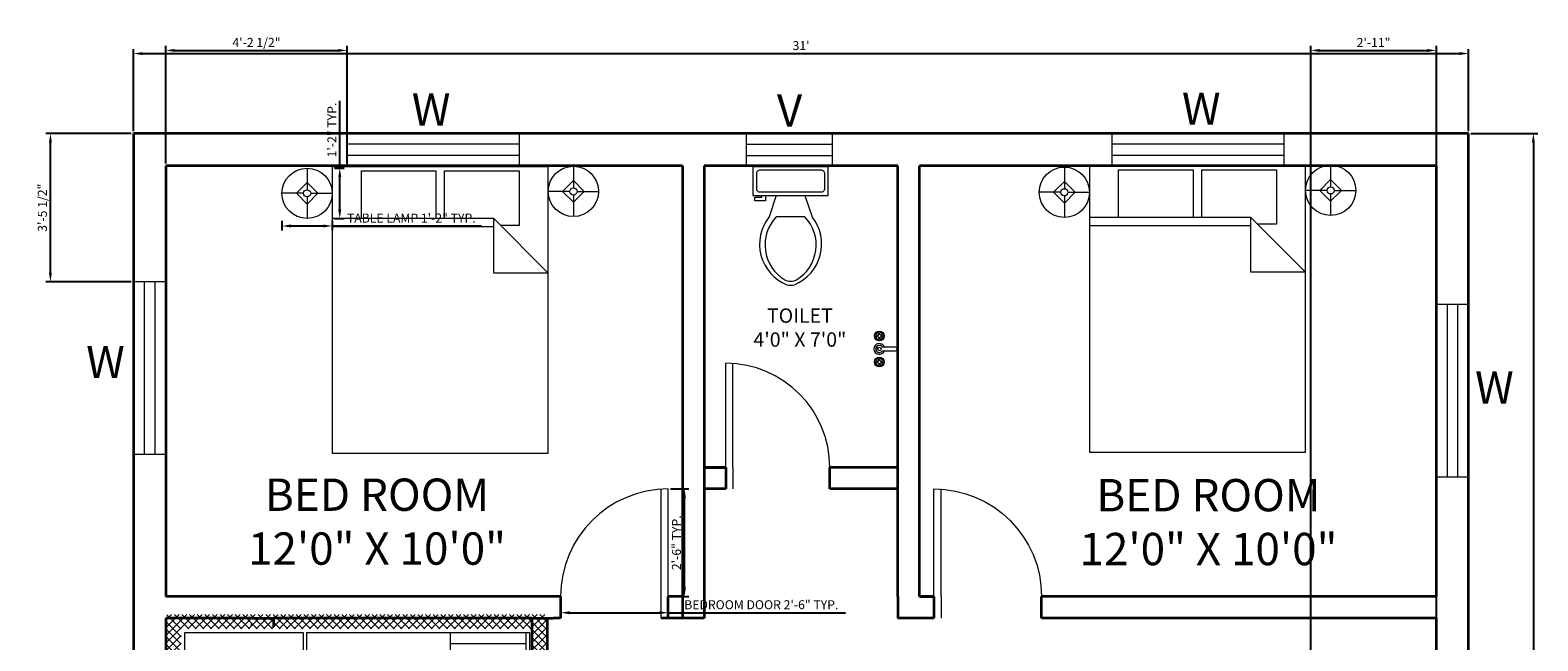
# Model space of a CAD drawing. Units: inches. Extents: x 1642 to 5612, y 1595 to 4064.
# Tile 6 of 6: x 2333 to 2754, y 1979 to 2149. Entities that reach past the tile are written whole.
import ezdxf

# ---------------------------------------------------------------- set-up
doc = ezdxf.new("R2010")
doc.units = ezdxf.units.IN
for name, color, linetype, lineweight in [('A-ANNO-DIMS', 2, 'Continuous', 18), ('A-ANNO-TEXT', 7, 'Continuous', 18), ('A-AREA-IDEN', 7, 'Continuous', 25), ('A-DOOR', 3, 'Continuous', 18), ('A-FLOR-FIXT', 9, 'Continuous', 18), ('A-FURN', 8, 'Continuous', 13), ('A-GLAZ', 4, 'Continuous', 18), ('A-WALL', 7, 'Continuous', 35)]:
    doc.layers.add(name, color=color, linetype=linetype, lineweight=lineweight)
doc.styles.get("Standard").update_dxf_attribs({"font": 'arial.ttf'})
doc.dimstyles.new('ISO-25', dxfattribs={"dimtxt": 2.5, "dimasz": 2.5, "dimexe": 1.25, "dimexo": 0.625, "dimtad": 1, "dimdec": 0, "dimlunit": 3, "dimtxsty": 'Standard', "dimcen": 2.5, "dimadec": 0, "dimazin": 0, "dimtfac": 1, "dimtdec": 0, "dimtmove": 0, "dimatfit": 3, "dimfxl": 1, "dimarcsym": 0})

# ---------------------------------------------------------------- blocks, each defined once
blk = doc.blocks.new('Kitchen Layout - 7 x 8 ft')
for p, q in [((-5, 81.32), (2.68, 89)), ((-5, 83.44), (0.56, 89)), ((-5, 85.56), (-1.56, 89)), ((-5, 87.68), (-3.68, 89)), ((-1, 84.97), (-5, 88.97)), ((1.09, 85), (-2.91, 89)), ((3.21, 85), (-0.79, 89)), ((0.81, 85), (4.81, 89)), ((5.34, 85), (1.34, 89)), ((2.93, 85), (6.93, 89)), ((7.46, 85), (3.46, 89)), ((5.05, 85), (9.05, 89)), ((9.58, 85), (5.58, 89)), ((7.17, 85), (11.17, 89)), ((11.7, 85), (7.7, 89)), ((9.29, 85), (13.29, 89)), ((13.82, 85), (9.82, 89)), ((11.41, 85), (15.41, 89)), ((15.94, 85), (11.94, 89)), ((13.53, 85), (17.53, 89)), ((18.06, 85), (14.06, 89)), ((15.65, 85), (19.65, 89)), ((20.18, 85), (16.18, 89)), ((17.78, 85), (21.78, 89)), ((22.31, 85), (18.31, 89)), ((19.9, 85), (23.9, 89)), ((24.43, 85), (20.43, 89)), ((22.02, 85), (26.02, 89)), ((26.55, 85), (22.55, 89)), ((24.14, 85), (28.14, 89)), ((28.67, 85), (24.67, 89)), ((26.26, 85), (30.26, 89)), ((30.79, 85), (26.79, 89)), ((28.38, 85), (32.38, 89)), ((32.91, 85), (28.91, 89)), ((30.5, 85), (34.5, 89)), ((35.03, 85), (31.03, 89)), ((32.63, 85), (36.63, 89)), ((37.16, 85), (33.16, 89)), ((34.75, 85), (38.75, 89)), ((39.28, 85), (35.28, 89)), ((36.87, 85), (40.87, 89)), ((41.4, 85), (37.4, 89)), ((38.99, 85), (42.99, 89)), ((43.52, 85), (39.52, 89)), ((41.11, 85), (45.11, 89)), ((45.64, 85), (41.64, 89)), ((43.23, 85), (47.23, 89)), ((47.76, 85), (43.76, 89)), ((45.35, 85), (49.35, 89)), ((49.88, 85), (45.88, 89)), ((47.47, 85), (51.47, 89)), ((52, 85), (48, 89)), ((49.6, 85), (53.6, 89)), ((54.13, 85), (50.13, 89)), ((51.72, 85), (55.72, 89)), ((56.25, 85), (52.25, 89)), ((53.84, 85), (57.84, 89)), ((58.37, 85), (54.37, 89)), ((55.96, 85), (59.96, 89)), ((60.49, 85), (56.49, 89)), ((58.08, 85), (62.08, 89)), ((62.61, 85), (58.61, 89)), ((60.2, 85), (64.2, 89)), ((64.73, 85), (60.73, 89)), ((62.32, 85), (66.32, 89)), ((66.85, 85), (62.85, 89)), ((64.45, 85), (68.45, 89)), ((68.97, 85), (64.97, 89)), ((66.57, 85), (70.57, 89)), ((71.1, 85), (67.1, 89)), ((68.69, 85), (72.69, 89)), ((73.22, 85), (69.22, 89)), ((70.81, 85), (74.81, 89)), ((75.34, 85), (71.34, 89)), ((72.93, 85), (76.93, 89)), ((77.46, 85), (73.46, 89)), ((75.05, 85), (79.05, 89)), ((79.58, 85), (75.58, 89)), ((77.17, 85), (81.17, 89)), ((81.7, 85), (77.7, 89)), ((79.29, 85), (83.29, 89)), ((83.82, 85), (79.82, 89)), ((81.42, 85), (85.42, 89)), ((85.95, 85), (81.95, 89)), ((83.54, 85), (87.54, 89)), ((88.07, 85), (84.07, 89)), ((85.66, 85), (89.66, 89)), ((90.19, 85), (86.19, 89)), ((87.78, 85), (91.78, 89)), ((92.31, 85), (88.31, 89)), ((89.9, 85), (93.9, 89)), ((94.43, 85), (90.43, 89)), ((92.02, 85), (96.02, 89)), ((96.55, 85), (92.55, 89)), ((94.14, 85), (98.14, 89)), ((101, 82.67), (94.67, 89)), ((96.27, 85), (100.27, 89)), ((101, 84.79), (96.79, 89)), ((101, 86.92), (98.92, 89)), ((-1, 82.85), (-5, 86.85)), ((-1, 80.73), (-5, 84.73)), ((97, 83.61), (101, 87.61)), ((97, 81.49), (101, 85.49)), ((101, 80.55), (97, 84.55)), ((-5, 79.19), (-1, 83.19)), ((-1, 78.61), (-5, 82.61)), ((-5, 77.07), (-1, 81.07)), ((-1, 76.49), (-5, 80.49)), ((34, 84), (96, 84)), ((34, 60), (34, 84)), ((74, 81), (95, 81)), ((96, 84), (96, 60)), ((97, 79.37), (101, 83.37)), ((101, 78.43), (97, 82.43)), ((97, 77.25), (101, 81.25)), ((101, 76.31), (97, 80.31)), ((-5, 74.95), (-1, 78.95)), ((-1, 74.36), (-5, 78.36)), ((-5, 72.83), (-1, 76.83)), ((-1, 72.24), (-5, 76.24)), ((97, 75.13), (101, 79.13)), ((101, 74.19), (97, 78.19)), ((97, 73.01), (101, 77.01)), ((101, 72.07), (97, 76.07)), ((-5, 70.71), (-1, 74.71)), ((-1, 70.12), (-5, 74.12)), ((-5, 68.59), (-1, 72.59)), ((-1, 68), (-5, 72)), ((97, 70.89), (101, 74.89)), ((101, 69.95), (97, 73.95)), ((97, 68.76), (101, 72.76)), ((101, 67.82), (97, 71.82)), ((-5, 66.47), (-1, 70.47)), ((-1, 65.88), (-5, 69.88)), ((-5, 64.35), (-1, 68.35)), ((-1, 63.76), (-5, 67.76)), ((97, 66.64), (101, 70.64)), ((101, 65.7), (97, 69.7)), ((97, 64.52), (101, 68.52)), ((101, 63.58), (97, 67.58)), ((-5, 62.22), (-1, 66.22)), ((-1, 61.64), (-5, 65.64)), ((-5, 60.1), (-1, 64.1)), ((-1, 59.52), (-5, 63.52)), ((97, 62.4), (101, 66.4)), ((101, 61.46), (97, 65.46)), ((97, 60.28), (101, 64.28)), ((100.34, 60), (97, 63.34)), ((-5, 57.98), (-1, 61.98)), ((-1, 57.39), (-5, 61.39)), ((-1.73, 56), (-5, 59.27)), ((-4.86, 56), (-1, 59.86)), ((10.4, 24), (45.9, 59.5)), ((18.88, 24), (54.38, 59.5)), ((27.37, 24), (62.87, 59.5)), ((33.03, 55.11), (37.41, 59.5)), ((96, 60), (34, 60)), ((35.85, 24), (71.35, 59.5)), ((76.2, 24), (40.7, 59.5)), ((84.68, 24), (49.18, 59.5)), ((93.17, 24), (57.67, 59.5)), ((96, 29.65), (66.15, 59.5)), ((80, 60), (80, 59)), ((82, 59), (82, 60)), ((87, 59), (87, 60)), ((89, 60), (89, 59)), ((98.22, 60), (97, 61.22)), ((98.84, 60), (101, 62.16)), ((100.96, 60), (101, 60.04)), ((-3.85, 56), (-5, 57.15)), ((-2.74, 56), (-1, 57.74)), ((0, 57), (33, 57)), ((0, 30.57), (24.43, 55)), ((0, 39.06), (15.94, 55)), ((0, 47.54), (7.46, 55)), ((1.91, 24), (32.91, 55)), ((33.77, 24), (2.77, 55)), ((42.26, 24), (11.26, 55)), ((50.74, 24), (19.74, 55)), ((59.23, 24), (28.23, 55)), ((31, 55), (31, 56)), ((32, 55), (31, 55)), ((32, 56), (32, 55)), ((67.71, 24), (33.68, 58.04)), ((44.34, 24), (77.84, 57.5)), ((52.82, 24), (86.32, 57.5)), ((61.31, 24), (96, 58.69)), ((96, 38.14), (76.64, 57.5)), ((96, 46.63), (85.13, 57.5)), ((96, 55.11), (93.57, 57.54)), ((25.29, 24), (0, 49.29)), ((69.79, 24), (96, 50.21)), ((16.8, 24), (0, 40.8)), ((78.28, 24), (96, 41.72)), ((8.32, 24), (0, 32.32)), ((86.76, 24), (96, 33.24)), ((-5, 21.92), (-2.92, 24)), ((-5, 19.8), (-1, 23.8)), ((-1, 19.21), (-5, 23.21)), ((-5, 17.68), (-1, 21.68)), ((-1, 17.09), (-5, 21.09)), ((-1, 21.33), (-3.67, 24)), ((-1, 23.45), (-1.55, 24)), ((0, 24), (96, 24)), ((0, 0), (0, 24)), ((95.25, 24), (96, 24.75)), ((96, 24), (96, 0)), ((97, 22.1), (98.9, 24)), ((97, 19.97), (101, 23.97)), ((101, 19.03), (97, 23.03)), ((97, 17.85), (101, 21.85)), ((101, 21.16), (98.16, 24)), ((101, 23.28), (100.28, 24)), ((-5, 15.55), (-1, 19.55)), ((-1, 14.97), (-5, 18.97)), ((-5, 13.43), (-1, 17.43)), ((-1, 12.85), (-5, 16.85)), ((47.25, 6.5), (47.25, 18.5)), ((48.75, 18.5), (48.75, 6.5)), ((101, 16.91), (97, 20.91)), ((97, 15.73), (101, 19.73)), ((101, 14.79), (97, 18.79)), ((97, 13.61), (101, 17.61)), ((-5, 11.31), (-1, 15.31)), ((-1, 10.73), (-5, 14.73)), ((-5, 9.19), (-1, 13.19)), ((-1, 8.6), (-5, 12.6)), ((101, 12.67), (97, 16.67)), ((97, 11.49), (101, 15.49)), ((101, 10.55), (97, 14.55)), ((97, 9.37), (101, 13.37)), ((-5, 7.07), (-1, 11.07)), ((-1, 6.48), (-5, 10.48)), ((-5, 4.95), (-1, 8.95)), ((101, 8.43), (97, 12.43)), ((97, 7.25), (101, 11.25)), ((101, 6.31), (97, 10.31)), ((97, 5.12), (101, 9.12)), ((-1, 4.36), (-5, 8.36)), ((-5, 2.83), (-1, 6.83)), ((-1, 2.24), (-5, 6.24)), ((-5, 0.71), (-1, 4.71)), ((101, 4.18), (97, 8.18)), ((97, 3), (101, 7)), ((101, 2.06), (97, 6.06)), ((97, 0.88), (101, 4.88)), ((-1, 0.12), (-5, 4.12)), ((-5, -1.42), (-1, 2.58)), ((2, -5), (-5, 2)), ((-5, -3.54), (-1, 0.46)), ((96, 0), (0, 0)), ((64, 4), (32, 4)), ((93.24, -5), (101, 2.76)), ((95.36, -5), (101, 0.64)), ((101, -0.06), (97, 3.94)), ((101, -2.18), (97, 1.82)), ((-0.12, -5), (-5, -0.12)), ((-2.25, -5), (-5, -2.25)), ((-4.34, -5), (-0.34, -1)), ((-2.22, -5), (1.78, -1)), ((-0.1, -5), (3.9, -1)), ((4.12, -5), (0.12, -1)), ((2.02, -5), (6.02, -1)), ((6.24, -5), (2.24, -1)), ((4.14, -5), (8.14, -1)), ((8.36, -5), (4.36, -1)), ((6.27, -5), (10.27, -1)), ((10.48, -5), (6.48, -1)), ((8.39, -5), (12.39, -1)), ((12.6, -5), (8.6, -1)), ((10.51, -5), (14.51, -1)), ((14.73, -5), (10.73, -1)), ((12.63, -5), (16.63, -1)), ((16.85, -5), (12.85, -1)), ((14.75, -5), (18.75, -1)), ((18.97, -5), (14.97, -1)), ((16.87, -5), (20.87, -1)), ((21.09, -5), (17.09, -1)), ((18.99, -5), (22.99, -1)), ((23.21, -5), (19.21, -1)), ((21.11, -5), (25.11, -1)), ((25.33, -5), (21.33, -1)), ((23.24, -5), (27.24, -1)), ((27.45, -5), (23.45, -1)), ((25.36, -5), (29.36, -1)), ((29.57, -5), (25.57, -1)), ((27.48, -5), (30, -2.48)), ((30, -3.3), (27.7, -1)), ((30, -1.18), (29.82, -1)), ((66, -2.54), (67.54, -1)), ((66, -4.66), (69.66, -1)), ((69.88, -5), (66, -1.12)), ((67.76, -5), (66, -3.24)), ((67.78, -5), (71.78, -1)), ((72, -5), (68, -1)), ((69.9, -5), (73.9, -1)), ((74.12, -5), (70.12, -1)), ((72.03, -5), (76.03, -1)), ((76.24, -5), (72.24, -1)), ((74.15, -5), (78.15, -1)), ((78.36, -5), (74.36, -1)), ((76.27, -5), (80.27, -1)), ((80.49, -5), (76.49, -1)), ((78.39, -5), (82.39, -1)), ((82.61, -5), (78.61, -1)), ((80.51, -5), (84.51, -1)), ((84.73, -5), (80.73, -1)), ((82.63, -5), (86.63, -1)), ((86.85, -5), (82.85, -1)), ((84.75, -5), (88.75, -1)), ((88.97, -5), (84.97, -1)), ((86.88, -5), (90.88, -1)), ((91.09, -5), (87.09, -1)), ((89, -5), (93, -1)), ((93.21, -5), (89.21, -1)), ((91.12, -5), (95.12, -1)), ((95.34, -5), (91.34, -1)), ((97.46, -5), (93.46, -1)), ((99.58, -5), (95.58, -1)), ((101, -4.3), (97, -0.3)), ((97.48, -5), (101, -1.48)), ((99.6, -5), (101, -3.6)), ((-4.37, -5), (-5, -4.37)), ((29.6, -5), (30, -4.6))]:
    blk.add_line(p, q)
for points in [[(0, 56), (0, 84), (33, 84), (33, 56)], [(74, 60), (74, 84), (95, 84), (95, 60)], [(76, 58), (76, 59), (93, 59), (93, 58)]]:
    blk.add_lwpolyline(points, close=True)
for points in [[(32, 1.5), (32, 19.5)], [(33.5, 21), (62.5, 21)], [(33.5, 6.5), (33.5, 18.5)], [(34.5, 19.5), (46.25, 19.5)], [(49.75, 19.5), (61.5, 19.5)], [(62.5, 18.5), (62.5, 6.5)], [(64, 19.5), (64, 1.5)], [(46.25, 5.5), (34.5, 5.5)], [(61.5, 5.5), (49.75, 5.5)], [(62.5, 0), (33.5, 0)]]:
    blk.add_lwpolyline(points)
for centre, radius in [((80, 75), 4), ((80, 75), 3), ((80, 75), 2), ((80, 75), 1), ((89, 75), 3), ((89, 75), 2), ((89, 75), 1), ((80, 66), 3), ((80, 66), 2), ((89, 66), 4), ((89, 66), 3), ((89, 66), 2), ((80, 66), 1), ((89, 66), 1), ((40.5, 12.5), 1), ((40.5, 12.5), 0.5), ((55.5, 12.5), 1), ((55.5, 12.5), 0.5)]:
    blk.add_circle(centre, radius)
for centre, radius, start, end in [((33.5, 19.5), 1.5, 90, 180), ((34.5, 18.5), 1, 90, 180), ((46.25, 18.5), 1, 0, 90), ((49.75, 18.5), 1, 90, 180), ((61.5, 18.5), 1, 0, 90), ((62.5, 19.5), 1.5, 0, 90), ((34.5, 6.5), 1, 180, 270), ((46.25, 6.5), 1, 270, 0), ((49.75, 6.5), 1, 180, 270), ((61.5, 6.5), 1, 270, 0), ((33.5, 1.5), 1.5, 180, 270), ((62.5, 1.5), 1.5, 270, 0)]:
    blk.add_arc(centre, radius, start, end)
blk = doc.blocks.new('Bed - Queen')
for p, q in [((0, -80.00003), (0, 0)), ((0, 0), (59.99999, 0)), ((59.99999, 0), (59.99999, -80.00003)), ((7.99999, -1.2), (28.79998, -1.2)), ((7.99999, -14.4), (7.99999, -1.2)), ((28.79998, -1.2), (28.79998, -14.4)), ((31.19999, -1.2), (51.99999, -1.2)), ((31.19999, -14.4), (31.19999, -1.2)), ((51.99999, -1.2), (51.99999, -16.4)), ((0, -14.4), (44.8, -14.4)), ((44.8, -16.8), (0, -16.8)), ((59.99999, -29.6), (44.8, -14.4)), ((44.8, -14.4), (44.8, -29.6)), ((51.99999, -16.4), (46.79936, -16.4)), ((44.8, -29.6), (59.99999, -29.6)), ((59.99999, -80.00003), (0, -80.00003))]:
    blk.add_line(p, q)
blk = doc.blocks.new('Lamp - Table')
for p, q in [((0, 7), (0, 1)), ((-1, 0), (-7, 0)), ((0, 3), (-3, 0)), ((-3, 0), (0, -3)), ((3, 0), (0, 3)), ((0, -3), (3, 0)), ((1, 0), (7, 0)), ((0, -1), (0, -7))]:
    blk.add_line(p, q)
for radius in [7, 1]:
    blk.add_circle((0, 0), radius)
blk = doc.blocks.new('Toilet - top')
for p, q in [((9.5, -6), (9.5, -2)), ((-8, -8.5), (-8, -8)), ((-7, -8), (-7, -9.5)), ((-4, -8), (-6, -14)), ((4, -8), (6, -14)), ((-10, -8.5), (-8, -8.5)), ((-10, -9.5), (-10, -8.5)), ((-7, -9.5), (-10, -9.5)), ((4, -14), (-4, -14))]:
    blk.add_line(p, q)
blk.add_lwpolyline([(10.5, -8), (10.5, 0), (-10.5, 0), (-10.5, -8)], close=True)
for points in [[(-9.5, -2), (-9.5, -6)], [(8.5, -1), (-8.5, -1)], [(-8.5, -7), (8.5, -7)]]:
    blk.add_lwpolyline(points)
for centre, radius, start, end in [((-8.62, -1.88), 0.884, 81.8699, 188.1301), ((8.62, -1.88), 0.884, 351.8699, 98.1301), ((-8.62, -6.12), 0.884, 171.8699, 278.1301), ((8.62, -6.12), 0.884, 261.8699, 8.1301), ((3.52, -21.58), 12.17, 141.4691, 247.9714), ((4.2, -21.82), 11.33, 136.3677, 238.9468), ((-3.52, -21.58), 12.17, 292.0284, 38.5307), ((-4.2, -21.82), 11.33, 301.053, 43.6321), ((0, -27.88), 4, 245.7318, 294.2682), ((0, -29), 4, 254.8605, 285.1395)]:
    blk.add_arc(centre, radius, start, end)
blk = doc.blocks.new('Faucet - Bathroom top')
for p, q in [((-4.107, 0.125), (-4.375, 0.125)), ((-3.75, 0.4788), (-3.75, 0.75)), ((-3.5, 0.482), (-3.5, 0.75)), ((-3.1461, 0.125), (-2.875, 0.125)), ((3.143, 0.125), (2.875, 0.125)), ((3.5, 0.4788), (3.5, 0.75)), ((3.75, 0.482), (3.75, 0.75)), ((4.1039, 0.125), (4.375, 0.125)), ((-4.1039, -0.125), (-4.375, -0.125)), ((-3.75, -0.4821), (-3.75, -0.75)), ((-3.5, -0.4789), (-3.5, -0.75)), ((-3.143, -0.125), (-2.875, -0.125)), ((-0.5, -0.8639), (-0.5, -4.5)), ((0.5, -4.5), (0.5, -0.8631)), ((3.1461, -0.125), (2.875, -0.125)), ((3.5, -0.4821), (3.5, -0.75)), ((3.75, -0.4789), (3.75, -0.75)), ((4.107, -0.125), (4.375, -0.125))]:
    blk.add_line(p, q)
for centre, radius in [((-3.625, 0), 1.375), ((-4.625, 0), 0.2795), ((-3.625, 0), 0.5), ((-3.625, 1), 0.2795), ((-2.625, 0), 0.2795), ((0, 0), 0.5), ((3.625, 0), 1.375), ((2.625, 0), 0.2795), ((3.625, 0), 0.5), ((3.625, 1), 0.2795), ((4.625, 0), 0.2795), ((-3.625, -1), 0.2795), ((3.625, -1), 0.2795)]:
    blk.add_circle(centre, radius)
for centre, radius, start, end in [((-3.625, 0), 1, 105.2407, 164.2093), ((-3.625, 0), 1, 16.44125, 74.07887), ((0, 0), 1.5, 289.6514, 250.3603), ((0, 0), 1, 300.3431, 239.7554), ((3.625, 0), 1, 106.12, 164.0884), ((3.625, 0), 1, 16.23422, 73.90469), ((-3.625, 0), 1, 196.2342, 253.9047), ((-3.625, 0), 1, 286.12, 344.0884), ((3.625, 0), 1, 196.4413, 254.0789), ((3.625, 0), 1, 285.2407, 344.2093), ((0, -4.5), 0.5, 180, 0)]:
    blk.add_arc(centre, radius, start, end)
blk = doc.blocks.new('*D14')
at = {"layer": 'A-ANNO-DIMS', "color": 0, "lineweight": -2, "transparency": 16777216}
for p, q in [((2362.27, 2121.26), (2362.27, 2144.16)), ((2364.77, 2142.91), (2731.77, 2142.91)), ((2734.27, 2121.26), (2734.27, 2144.16))]:
    blk.add_line(p, q, dxfattribs=at)
at = {"layer": 'A-ANNO-DIMS', "color": 0, "transparency": 16777216}
for points in [[(2364.77, 2143.33), (2364.77, 2142.49), (2362.27, 2142.91)], [(2731.77, 2143.33), (2731.77, 2142.49), (2734.27, 2142.91)]]:
    blk.add_solid(points, dxfattribs=at)
at = {"layer": 'Defpoints', "color": 0, "transparency": 16777216}
for p in [(2734.27, 2142.91), (2362.27, 2120.64), (2734.27, 2120.64)]:
    blk.add_point(p, dxfattribs=at)
at = {"layer": 'A-ANNO-DIMS', "color": 0, "transparency": 16777216, "insert": (2548.27, 2144.81), "char_height": 2.5, "attachment_point": 5}
blk.add_mtext("31'", dxfattribs=at)
blk = doc.blocks.new('*D15')
at = {"layer": 'A-ANNO-DIMS', "color": 0, "lineweight": -2, "transparency": 16777216}
for p, q in [((2734.9, 2120.64), (2753.55, 2120.64)), ((2752.3, 2118.14), (2752.3, 1739.14)), ((2734.9, 1736.64), (2753.55, 1736.64))]:
    blk.add_line(p, q, dxfattribs=at)
at = {"layer": 'A-ANNO-DIMS', "color": 0, "transparency": 16777216}
for points in [[(2751.88, 2118.14), (2752.72, 2118.14), (2752.3, 2120.64)], [(2751.88, 1739.14), (2752.72, 1739.14), (2752.3, 1736.64)]]:
    blk.add_solid(points, dxfattribs=at)
at = {"layer": 'Defpoints', "color": 0, "transparency": 16777216}
for p in [(2734.27, 2120.64), (2734.27, 1736.64), (2752.3, 1736.64)]:
    blk.add_point(p, dxfattribs=at)
at = {"layer": 'A-ANNO-DIMS', "color": 0, "transparency": 16777216, "insert": (2750.4, 1928.64), "char_height": 2.5, "attachment_point": 5, "rotation": 90}
blk.add_mtext("32'", dxfattribs=at)
blk = doc.blocks.new('WIN-48x9')
for p, q in [((0, 48), (0, 0)), ((9, 48), (0, 48)), ((3, 48), (3, 0)), ((6, 0), (6, 48)), ((9, 0), (9, 48)), ((0, 0), (9, 0))]:
    blk.add_line(p, q)
blk = doc.blocks.new('VENT-24x9')
for p, q in [((9, 24), (0, 24)), ((0, 24), (0, 0)), ((3, 24), (3, 0)), ((6, 0), (6, 24)), ((9, 0), (9, 24)), ((9, 0), (0, 0))]:
    blk.add_line(p, q)
blk = doc.blocks.new('DOOR-SWING-29')
for p, q in [((0, 29), (29, 29)), ((0, 27), (29, 27))]:
    blk.add_line(p, q)
blk.add_arc((0, 29), 29, 270, 0)
blk = doc.blocks.new('DOOR-SWING-30')
for p, q in [((28, 0), (28, 30)), ((30, 0), (30, 30))]:
    blk.add_line(p, q)
blk.add_arc((30, 0), 30, 90, 180)
blk = doc.blocks.new('*D26')
at = {"layer": 'A-ANNO-DIMS', "color": 0, "lineweight": -2, "transparency": 16777216}
for p, q in [((2403.64, 2096.35), (2403.64, 2093.63)), ((2417.64, 2096.35), (2417.64, 2093.63)), ((2406.14, 2094.88), (2415.14, 2094.88)), ((2417.64, 2094.88), (2459.21, 2094.88))]:
    blk.add_line(p, q, dxfattribs=at)
at = {"layer": 'A-ANNO-DIMS', "color": 0, "transparency": 16777216}
for points in [[(2406.14, 2095.3), (2406.14, 2094.46), (2403.64, 2094.88)], [(2415.14, 2095.3), (2415.14, 2094.46), (2417.64, 2094.88)]]:
    blk.add_solid(points, dxfattribs=at)
at = {"layer": 'Defpoints', "color": 0, "transparency": 16777216}
for p in [(2403.64, 2096.98), (2417.64, 2096.98), (2417.64, 2094.88)]:
    blk.add_point(p, dxfattribs=at)
at = {"layer": 'A-ANNO-DIMS', "color": 0, "transparency": 16777216, "insert": (2439.67, 2096.76), "char_height": 2.5, "attachment_point": 5}
blk.add_mtext('TABLE LAMP 1\'-2" TYP.', dxfattribs=at)
blk = doc.blocks.new('*D27')
at = {"layer": 'A-ANNO-DIMS', "color": 0, "lineweight": -2, "transparency": 16777216}
for p, q in [((2419.74, 2110.98), (2419.74, 2129.73)), ((2418.26, 2110.98), (2420.99, 2110.98)), ((2419.74, 2099.48), (2419.74, 2108.48)), ((2418.26, 2096.98), (2420.99, 2096.98))]:
    blk.add_line(p, q, dxfattribs=at)
at = {"layer": 'A-ANNO-DIMS', "color": 0, "transparency": 16777216}
for points in [[(2419.32, 2108.48), (2420.16, 2108.48), (2419.74, 2110.98)], [(2419.32, 2099.48), (2420.16, 2099.48), (2419.74, 2096.98)]]:
    blk.add_solid(points, dxfattribs=at)
at = {"layer": 'Defpoints', "color": 0, "transparency": 16777216}
for p in [(2417.64, 2110.98), (2419.74, 2110.98), (2417.64, 2096.98)]:
    blk.add_point(p, dxfattribs=at)
at = {"layer": 'A-ANNO-DIMS', "color": 0, "transparency": 16777216, "insert": (2417.86, 2121.61), "char_height": 2.5, "attachment_point": 5, "rotation": 90}
blk.add_mtext('1\'-2" TYP.', dxfattribs=at)
blk = doc.blocks.new('*D52')
at = {"layer": 'A-ANNO-DIMS', "color": 0, "lineweight": -2, "transparency": 16777216}
for p, q in [((2481.27, 1991.01), (2481.27, 1985.89)), ((2483.77, 1987.14), (2508.77, 1987.14)), ((2511.27, 1991.01), (2511.27, 1985.89)), ((2511.27, 1987.14), (2560.61, 1987.14))]:
    blk.add_line(p, q, dxfattribs=at)
at = {"layer": 'A-ANNO-DIMS', "color": 0, "transparency": 16777216}
for points in [[(2483.77, 1987.55), (2483.77, 1986.72), (2481.27, 1987.14)], [(2508.77, 1987.55), (2508.77, 1986.72), (2511.27, 1987.14)]]:
    blk.add_solid(points, dxfattribs=at)
at = {"layer": 'Defpoints', "color": 0, "transparency": 16777216}
for p in [(2481.27, 1991.64), (2511.27, 1991.64), (2511.27, 1987.14)]:
    blk.add_point(p, dxfattribs=at)
at = {"layer": 'A-ANNO-DIMS', "color": 0, "transparency": 16777216, "insert": (2537.19, 1989.05), "char_height": 2.5, "attachment_point": 5}
blk.add_mtext('BEDROOM DOOR 2\'-6" TYP.', dxfattribs=at)
blk = doc.blocks.new('*D53')
at = {"layer": 'A-ANNO-DIMS', "color": 0, "lineweight": -2, "transparency": 16777216}
for p, q in [((2511.9, 2021.64), (2517.02, 2021.64)), ((2515.77, 1994.14), (2515.77, 2019.14)), ((2511.9, 1991.64), (2517.02, 1991.64))]:
    blk.add_line(p, q, dxfattribs=at)
at = {"layer": 'A-ANNO-DIMS', "color": 0, "transparency": 16777216}
for points in [[(2515.36, 2019.14), (2516.19, 2019.14), (2515.77, 2021.64)], [(2515.36, 1994.14), (2516.19, 1994.14), (2515.77, 1991.64)]]:
    blk.add_solid(points, dxfattribs=at)
at = {"layer": 'Defpoints', "color": 0, "transparency": 16777216}
for p in [(2511.27, 2021.64), (2515.77, 2021.64), (2511.27, 1991.64)]:
    blk.add_point(p, dxfattribs=at)
at = {"layer": 'A-ANNO-DIMS', "color": 0, "transparency": 16777216, "insert": (2513.87, 2006.64), "char_height": 2.5, "attachment_point": 5, "rotation": 90}
blk.add_mtext('2\'-6" TYP.', dxfattribs=at)
blk = doc.blocks.new('*D62')
at = {"layer": 'A-ANNO-DIMS', "color": 0, "lineweight": -2, "transparency": 16777216}
for p, q in [((2371.27, 2112.26), (2371.27, 2145.04)), ((2373.77, 2143.79), (2419.31, 2143.79)), ((2421.81, 2112.26), (2421.81, 2145.04))]:
    blk.add_line(p, q, dxfattribs=at)
at = {"layer": 'A-ANNO-DIMS', "color": 0, "transparency": 16777216}
for points in [[(2373.77, 2144.2), (2373.77, 2143.37), (2371.27, 2143.79)], [(2419.31, 2144.2), (2419.31, 2143.37), (2421.81, 2143.79)]]:
    blk.add_solid(points, dxfattribs=at)
at = {"layer": 'Defpoints', "color": 0, "transparency": 16777216}
for p in [(2421.81, 2143.79), (2371.27, 2111.64), (2421.81, 2111.64)]:
    blk.add_point(p, dxfattribs=at)
at = {"layer": 'A-ANNO-DIMS', "color": 0, "transparency": 16777216, "insert": (2396.54, 2145.7), "char_height": 2.5, "attachment_point": 5}
blk.add_mtext('4\'-2 1/2"', dxfattribs=at)
blk = doc.blocks.new('*D63')
at = {"layer": 'A-ANNO-DIMS', "color": 0, "lineweight": -2, "transparency": 16777216}
for p, q in [((2361.65, 2120.64), (2337.87, 2120.64)), ((2339.12, 2081.8), (2339.12, 2118.14)), ((2361.65, 2079.3), (2337.87, 2079.3))]:
    blk.add_line(p, q, dxfattribs=at)
at = {"layer": 'A-ANNO-DIMS', "color": 0, "transparency": 16777216}
for points in [[(2338.71, 2118.14), (2339.54, 2118.14), (2339.12, 2120.64)], [(2338.71, 2081.8), (2339.54, 2081.8), (2339.12, 2079.3)]]:
    blk.add_solid(points, dxfattribs=at)
at = {"layer": 'Defpoints', "color": 0, "transparency": 16777216}
for p in [(2339.12, 2120.64), (2362.27, 2120.64), (2362.27, 2079.3)]:
    blk.add_point(p, dxfattribs=at)
at = {"layer": 'A-ANNO-DIMS', "color": 0, "transparency": 16777216, "insert": (2337.2, 2099.97), "char_height": 2.5, "attachment_point": 5, "rotation": 90}
blk.add_mtext('3\'-5 1/2"', dxfattribs=at)
blk = doc.blocks.new('*D65')
at = {"layer": 'A-ANNO-DIMS', "color": 0, "lineweight": -2, "transparency": 16777216}
for p, q in [((2690.27, 1746.26), (2690.27, 2145.04)), ((2692.77, 2143.79), (2722.77, 2143.79)), ((2725.27, 1746.26), (2725.27, 2145.04))]:
    blk.add_line(p, q, dxfattribs=at)
at = {"layer": 'A-ANNO-DIMS', "color": 0, "transparency": 16777216}
for points in [[(2692.77, 2144.2), (2692.77, 2143.37), (2690.27, 2143.79)], [(2722.77, 2144.2), (2722.77, 2143.37), (2725.27, 2143.79)]]:
    blk.add_solid(points, dxfattribs=at)
at = {"layer": 'Defpoints', "color": 0, "transparency": 16777216}
for p in [(2725.27, 2143.79), (2690.27, 1745.64), (2725.27, 1745.64)]:
    blk.add_point(p, dxfattribs=at)
at = {"layer": 'A-ANNO-DIMS', "color": 0, "transparency": 16777216, "insert": (2707.77, 2145.67), "char_height": 2.5, "attachment_point": 5}
blk.add_mtext('2\'-11"', dxfattribs=at)

msp = doc.modelspace()

# ---------------------------------------------------------------- linework, layer by layer
at = {"layer": 'A-DOOR'}
for p, q in [((2529.27, 2027.64), (2529.27, 2021.64)), ((2509.27, 1985.64), (2509.27, 1991.64)), ((2587.27, 1991.64), (2587.27, 1985.64))]:
    msp.add_line(p, q, dxfattribs=at)
at = {"layer": 'A-WALL'}
for p, q in [((2362.27, 2120.64), (2362.27, 1736.64)), ((2734.27, 2120.64), (2362.27, 2120.64)), ((2734.27, 1736.64), (2734.27, 2120.64)), ((2371.27, 2111.64), (2371.27, 1991.64)), ((2515.27, 2111.64), (2371.27, 2111.64)), ((2515.27, 2111.64), (2515.27, 1991.64)), ((2521.27, 2111.64), (2521.27, 1991.64)), ((2575.27, 2111.64), (2521.27, 2111.64)), ((2575.27, 1991.64), (2575.27, 2111.64)), ((2725.27, 2111.64), (2581.27, 2111.64)), ((2581.27, 1991.64), (2581.27, 2111.64)), ((2725.27, 1991.64), (2725.27, 2111.64)), ((2521.27, 2027.64), (2527.27, 2027.64)), ((2527.27, 2027.64), (2521.27, 2027.64)), ((2527.27, 2027.64), (2527.27, 2021.64)), ((2575.27, 2027.64), (2556.27, 2027.64)), ((2556.27, 2021.64), (2556.27, 2027.64)), ((2527.27, 2021.64), (2521.27, 2021.64)), ((2575.27, 2021.64), (2556.27, 2021.64)), ((2481.27, 1991.64), (2371.27, 1991.64)), ((2481.27, 1991.64), (2481.27, 1985.64)), ((2515.27, 1991.64), (2511.27, 1991.64)), ((2511.27, 1985.64), (2511.27, 1991.64)), ((2511.27, 1985.64), (2511.27, 1991.64)), ((2515.27, 1991.64), (2515.27, 1985.64)), ((2521.27, 1991.64), (2521.27, 1985.63)), ((2575.27, 1991.64), (2575.27, 1985.64)), ((2581.27, 1991.64), (2585.27, 1991.64)), ((2585.27, 1991.64), (2581.27, 1991.64)), ((2585.27, 1991.64), (2585.27, 1985.64)), ((2725.27, 1991.64), (2615.27, 1991.64)), ((2615.27, 1985.64), (2615.27, 1991.64)), ((2395.27, 1985.64), (2371.27, 1985.64)), ((2371.27, 1985.64), (2371.27, 1894.64)), ((2395.27, 1985.64), (2401.27, 1985.64)), ((2395.27, 1984.09), (2395.27, 1983.55)), ((2401.27, 1985.64), (2401.27, 1983.18)), ((2473.27, 1985.64), (2401.27, 1985.64)), ((2473.27, 1985.64), (2473.27, 1956.89)), ((2473.27, 1985.64), (2479.27, 1985.64)), ((2477.56, 1985.23), (2477.56, 1956.89)), ((2481.27, 1985.64), (2479.27, 1985.64)), ((2515.27, 1985.64), (2509.27, 1985.64)), ((2515.27, 1985.64), (2511.27, 1985.64)), ((2520.91, 1985.64), (2511.27, 1985.64)), ((2515.27, 1985.64), (2515.27, 1985.64)), ((2521.27, 1985.63), (2520.91, 1985.64)), ((2585.27, 1985.64), (2575.27, 1985.64)), ((2725.27, 1985.64), (2615.27, 1985.64)), ((2725.27, 1894.64), (2725.27, 1985.64))]:
    msp.add_line(p, q, dxfattribs=at)

# ---------------------------------------------------------------- block references
at = {"layer": 'A-DOOR', "rotation": 89.99999999999895}
msp.add_blockref('DOOR-SWING-29', (2556.27, 2027.64), dxfattribs=at)
at = {"layer": 'A-DOOR'}
msp.add_blockref('DOOR-SWING-30', (2481.27, 1991.64), dxfattribs=at)
at = {"layer": 'A-DOOR', "extrusion": (0, 0, -1), "zscale": -1}
msp.add_blockref('DOOR-SWING-30', (-2615.27, 1991.64), dxfattribs=at)
at = {"layer": 'A-FLOR-FIXT'}
for name, p in [('Toilet - top', (2545.35, 2111.39)), ('Kitchen Layout - 7 x 8 ft', (2376.56, 1897.61))]:
    msp.add_blockref(name, p, dxfattribs=at)
at = {"layer": 'A-FLOR-FIXT', "rotation": 89.99999999999999}
msp.add_blockref('Faucet - Bathroom top', (2570.06, 2060.62), dxfattribs=at)
at = {"layer": 'A-FURN'}
for name, p in [('Lamp - Table', (2410.64, 2103.98)), ('Bed - Queen', (2417.75, 2111.46)), ('Lamp - Table', (2484.84, 2104.51)), ('Lamp - Table', (2621.62, 2104.27)), ('Bed - Queen', (2628.73, 2111.75)), ('Lamp - Table', (2695.82, 2104.8))]:
    msp.add_blockref(name, p, dxfattribs=at)
at = {"layer": 'A-GLAZ'}
for name, p, rotation in [('WIN-48x9', (2421.81, 2120.64), 269.9999999999988), ('VENT-24x9', (2556.93, 2111.55), 90.00000000000072), ('WIN-48x9', (2634.84, 2120.64), 269.999999999999)]:
    msp.add_blockref(name, p, dxfattribs=dict(at, rotation=rotation))
for p in [(2362.27, 2031.31), (2725.27, 2025.03)]:
    msp.add_blockref('WIN-48x9', p, dxfattribs=at)

# ---------------------------------------------------------------- texts
at = {"layer": 'A-ANNO-TEXT', "char_height": 9, "attachment_point": 1}
for s, width, insert in [('\\pxqc;W', 122.7897, (2383.8, 2131.84)), ('\\pxqc;V', 37.3133, (2526.4, 2131.59)), ('\\pxqc;W', 122.7897, (2598.38, 2132.06)), ('\\pxqc;W', 122.7897, (2293.07, 2061.49)), ('\\pxqc;W', 122.7897, (2680.06, 2054.38))]:
    msp.add_mtext_dynamic_manual_height_columns(s, width=width, gutter_width=12.5, heights=[0], dxfattribs=dict(at, insert=insert))
at = {"layer": 'A-AREA-IDEN', "attachment_point": 1}
for s, width, insert, char_height in [('\\pxqc;TOILET\\P4\'0" X 7\'0"', 48, (2523.94, 2071.91), 4), ('\\pxqc;BED ROOM \\P12\'0" X 10\'0"', 95.4247, (2382.41, 2024.52), 9), ('\\pxqc;BED ROOM \\P12\'0" X 10\'0"', 95.4247, (2614.07, 2024.39), 9)]:
    msp.add_mtext_dynamic_manual_height_columns(s, width=width, gutter_width=12.5, heights=[0], dxfattribs=dict(at, insert=insert, char_height=char_height))

# ---------------------------------------------------------------- dimensions: what is measured, and where the dimension line sits
at = {"layer": 'A-ANNO-DIMS'}
for base, p1, p2, override, picture, middle in [((2421.81, 2143.79), (2371.27, 2111.64), (2421.81, 2111.64), {"dimdec": 1, "dimlfac": 1, "dimrnd": 0, "dimzin": 1, "dimdsep": 46, "dimlunit": 4, "dimfrac": 2}, '*D62', (2396.54, 2145.7)), ((2725.27, 2143.79), (2690.27, 1745.64), (2725.27, 1745.64), {"dimdec": 1, "dimlfac": 1, "dimrnd": 0, "dimzin": 1, "dimdsep": 46, "dimlunit": 4, "dimfrac": 2}, '*D65', (2707.77, 2145.67)), ((2734.27, 2142.91), (2362.27, 2120.64), (2734.27, 2120.64), {"dimclrd": 0, "dimclre": 0, "dimclrt": 0}, '*D14', (2548.27, 2144.81))]:
    dim = msp.add_linear_dim(base=base, p1=p1, p2=p2, dimstyle='ISO-25', override=override, dxfattribs=at)
    dim.commit()
    dim.dimension.update_dxf_attribs({"geometry": picture, "text_midpoint": middle})
for base, p1, p2, picture, middle in [((2419.74, 2110.98), (2417.64, 2096.98), (2417.64, 2110.98), '*D27', (2417.86, 2121.61)), ((2515.77, 2021.64), (2511.27, 1991.64), (2511.27, 2021.64), '*D53', (2513.87, 2006.64))]:
    dim = msp.add_linear_dim(base=base, p1=p1, p2=p2, angle=90, text='<> TYP.', dimstyle='ISO-25', override={"dimdec": 1, "dimlfac": 1, "dimrnd": 0, "dimzin": 1, "dimdsep": 46, "dimlunit": 4, "dimfrac": 2}, dxfattribs=at)
    dim.commit()
    dim.dimension.update_dxf_attribs({"geometry": picture, "text_midpoint": middle})
for base, p1, p2, override, picture, middle in [((2339.12, 2120.64), (2362.27, 2079.3), (2362.27, 2120.64), {"dimdec": 1, "dimlfac": 1, "dimrnd": 0, "dimzin": 1, "dimdsep": 46, "dimlunit": 4, "dimfrac": 2}, '*D63', (2337.2, 2099.97)), ((2752.3, 1736.64), (2734.27, 2120.64), (2734.27, 1736.64), {"dimclrd": 0, "dimclre": 0, "dimclrt": 0}, '*D15', (2750.4, 1928.64))]:
    dim = msp.add_linear_dim(base=base, p1=p1, p2=p2, angle=90, dimstyle='ISO-25', override=override, dxfattribs=at)
    dim.commit()
    dim.dimension.update_dxf_attribs({"geometry": picture, "text_midpoint": middle})
for base, p1, p2, text, picture, middle in [((2417.64, 2094.88), (2403.64, 2096.98), (2417.64, 2096.98), 'TABLE LAMP <> TYP.', '*D26', (2439.67, 2096.76)), ((2511.27, 1987.14), (2481.27, 1991.64), (2511.27, 1991.64), 'BEDROOM DOOR <> TYP.', '*D52', (2537.19, 1989.05))]:
    dim = msp.add_linear_dim(base=base, p1=p1, p2=p2, text=text, dimstyle='ISO-25', override={"dimdec": 1, "dimlfac": 1, "dimrnd": 0, "dimzin": 1, "dimdsep": 46, "dimlunit": 4, "dimfrac": 2}, dxfattribs=at)
    dim.commit()
    dim.dimension.update_dxf_attribs({"geometry": picture, "text_midpoint": middle})

doc.saveas('drawing.dxf')
